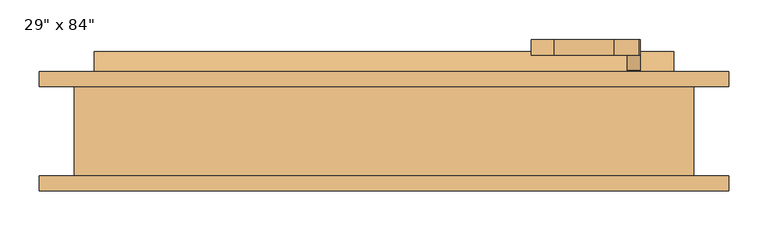
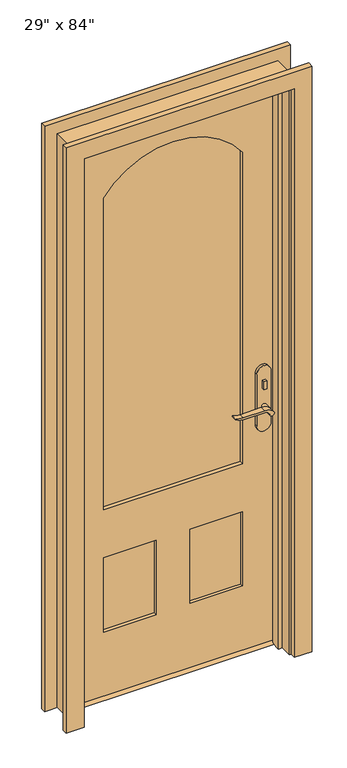
"""IFC4 building model written with IfcOpenShell, lengths in millimetres: door geometry."""

from ifc_helpers import new_model, si_unit, point, frame, frame_2d, origin, place, context, project, spatial, polyline, circle_curve, trimmed, segment, composite_curve, outline, extrude, faceted_brep, source, transform, mapped, element, save


def door_b81be692(model_context):
    return source(origin(), model_context, "Body", "SolidModel", [
        extrude(outline(polyline([(38.1, 12.7), (73.025, 12.7), (98.425, 0.0), (12.7, 0.0), (38.1, 12.7)])), frame((-368.3, 0.0, 0.0), z_axis=(1.0, 0.0, 0.0), x_axis=(0.0, 1.0, 0.0)), (0.0, 0.0, 1.0), 736.6),
        extrude(outline(polyline([(322.5, -0.95), (312.5, -0.95), (312.5, 9.05), (322.5, 9.05), (322.5, -0.95)])), frame((0.0, 0.0, 981.9), z_axis=(0.0, 0.0, 1.0), x_axis=(1.0, 0.0, 0.0)), (0.0, 0.0, 1.0), 30.0),
        extrude(outline(composite_curve([segment(trimmed(circle_curve(frame_2d((996.9, 317.5)), 8.0), [point((996.9, 309.5))], [point((996.9, 325.5))], False, "CARTESIAN"), True, "CONTINUOUS"), segment(trimmed(circle_curve(frame_2d((996.9, 317.5)), 8.0), [point((996.9, 325.5))], [point((996.9, 309.5))], False, "CARTESIAN"), True, "CONTINUOUS")], self_intersect=False)), frame((0.0, 63.975, 0.0), z_axis=(0.0, 1.0, 0.0), x_axis=(0.0, 0.0, 1.0)), (0.0, 0.0, 1.0), 10.0),
        extrude(outline(composite_curve([segment(trimmed(circle_curve(frame_2d((897.1555521, 293.8324871)), 37.2832219), [point((919.0523287, 324.0081363))], [point((934.4, 292.1325667))], False, "CARTESIAN"), True, "CONTINUOUS"), segment(polyline([(934.4, 292.1325667), (934.4, 215.8564091)]), True, "CONTINUOUS"), segment(trimmed(circle_curve(frame_2d((1017.6850638, 215.9227909)), 83.2850902), [point((934.4, 215.8564091))], [point((939.4, 187.5))], True, "CARTESIAN"), True, "CONTINUOUS"), segment(polyline([(939.4, 187.5), (936.6135558, 187.5)]), True, "CONTINUOUS"), segment(trimmed(circle_curve(frame_2d((986.6709207, 219.4396612)), 59.3791355), [point((936.6135558, 187.5))], [point((927.4, 215.8564091))], False, "CARTESIAN"), True, "CONTINUOUS"), segment(polyline([(927.4, 215.8564091), (927.4, 292.1138099)]), True, "CONTINUOUS"), segment(trimmed(circle_curve(frame_2d((909.2738613, 292.1138099)), 18.1261387), [point((927.4, 292.1138099))], [point((914.4, 309.5))], True, "CARTESIAN"), True, "CONTINUOUS"), segment(trimmed(circle_curve(frame_2d((914.4, 317.5)), 8.0), [point((914.4, 309.5))], [point((919.0523287, 324.0081363))], False, "CARTESIAN"), True, "CONTINUOUS")], self_intersect=False)), frame((0.0, -40.95, 0.0), z_axis=(0.0, 1.0, 0.0), x_axis=(0.0, 0.0, 1.0)), (0.0, 0.0, 1.0), 20.0),
        extrude(outline(composite_curve([segment(trimmed(circle_curve(frame_2d((914.4, 317.5)), 8.0), [point((914.3999903, 309.5))], [point((919.0523287, 324.0081363))], False, "CARTESIAN"), True, "CONTINUOUS"), segment(trimmed(circle_curve(frame_2d((897.1555521, 293.8324871)), 37.2832219), [point((919.0523287, 324.0081363))], [point((934.4, 292.1325667))], False, "CARTESIAN"), True, "CONTINUOUS"), segment(polyline([(934.4, 292.1325667), (934.4, 215.8564091)]), True, "CONTINUOUS"), segment(trimmed(circle_curve(frame_2d((1017.6850638, 215.9227909)), 83.2850902), [point((934.4, 215.8564091))], [point((939.4, 187.5))], True, "CARTESIAN"), True, "CONTINUOUS"), segment(polyline([(939.4, 187.5), (936.6135558, 187.5)]), True, "CONTINUOUS"), segment(trimmed(circle_curve(frame_2d((986.6709207, 219.4396612)), 59.3791355), [point((936.6135558, 187.5))], [point((927.4, 215.8564091))], False, "CARTESIAN"), True, "CONTINUOUS"), segment(polyline([(927.4, 215.8564091), (927.4, 292.1138122)]), True, "CONTINUOUS"), segment(trimmed(circle_curve(frame_2d((909.2738682, 292.1138122)), 18.1261318), [point((927.4, 292.1138122))], [point((914.3999903, 309.5))], True, "CARTESIAN"), True, "CONTINUOUS")], self_intersect=False)), frame((0.0, 93.975, 0.0), z_axis=(0.0, 1.0, 0.0), x_axis=(0.0, 0.0, 1.0)), (0.0, 0.0, 1.0), 20.0),
        extrude(outline(composite_curve([segment(trimmed(circle_curve(frame_2d((914.4, 317.5)), 8.0), [point((914.4, 309.5))], [point((914.4, 325.5))], False, "CARTESIAN"), True, "CONTINUOUS"), segment(trimmed(circle_curve(frame_2d((914.4, 317.5)), 8.0), [point((914.4, 325.5))], [point((914.4, 309.5))], False, "CARTESIAN"), True, "CONTINUOUS")], self_intersect=False)), frame((0.0, -20.95, 0.0), z_axis=(0.0, 1.0, 0.0), x_axis=(0.0, 0.0, 1.0)), (0.0, 0.0, 1.0), 30.0),
        extrude(outline(composite_curve([segment(trimmed(circle_curve(frame_2d((914.4, 317.5)), 8.0), [point((914.4, 309.5))], [point((914.4, 325.5))], False, "CARTESIAN"), True, "CONTINUOUS"), segment(trimmed(circle_curve(frame_2d((914.4, 317.5)), 8.0), [point((914.4, 325.5))], [point((914.4, 309.5))], False, "CARTESIAN"), True, "CONTINUOUS")], self_intersect=False)), frame((0.0, 63.975, 0.0), z_axis=(0.0, 1.0, 0.0), x_axis=(0.0, 0.0, 1.0)), (0.0, 0.0, 1.0), 30.0),
        extrude(outline(composite_curve([segment(polyline([(844.4, 342.5), (1039.4, 342.5)]), True, "CONTINUOUS"), segment(trimmed(circle_curve(frame_2d((1039.4, 317.5)), 25.0), [point((1039.4, 342.5))], [point((1039.4, 292.5))], False, "CARTESIAN"), True, "CONTINUOUS"), segment(polyline([(1039.4, 292.5), (844.4, 292.5)]), True, "CONTINUOUS"), segment(trimmed(circle_curve(frame_2d((844.4, 317.5)), 25.0), [point((844.4, 292.5))], [point((844.4, 342.5))], False, "CARTESIAN"), True, "CONTINUOUS")], self_intersect=False)), frame((0.0, 9.05, 0.0), z_axis=(0.0, 1.0, 0.0), x_axis=(0.0, 0.0, 1.0)), (0.0, 0.0, 1.0), 10.0),
        extrude(outline(composite_curve([segment(polyline([(844.4, 342.5), (1039.4, 342.5)]), True, "CONTINUOUS"), segment(trimmed(circle_curve(frame_2d((1039.4, 317.5)), 25.0), [point((1039.4, 342.5))], [point((1039.4, 292.5))], False, "CARTESIAN"), True, "CONTINUOUS"), segment(polyline([(1039.4, 292.5), (844.4, 292.5)]), True, "CONTINUOUS"), segment(trimmed(circle_curve(frame_2d((844.4, 317.5)), 25.0), [point((844.4, 292.5))], [point((844.4, 342.5))], False, "CARTESIAN"), True, "CONTINUOUS")], self_intersect=False)), frame((0.0, 53.975, 0.0), z_axis=(0.0, 1.0, 0.0), x_axis=(0.0, 0.0, 1.0)), (0.0, 0.0, 1.0), 10.0),
        faceted_brep([(393.7, 53.975, 0.0), (393.7, -60.325, 0.0), (368.3, -60.325, 0.0), (368.3, -15.875, 0.0), (355.6, -15.875, 0.0), (355.6, 19.05, 0.0), (368.3, 19.05, 0.0), (368.3, 53.975, 0.0), (393.7, 53.975, 2159.0), (393.7, -60.325, 2159.0), (-393.7, -60.325, 2159.0), (-393.7, -60.325, 0.0), (-368.3, -60.325, 0.0), (-368.3, -60.325, 2133.6), (368.3, -60.325, 2133.6), (368.3, -15.875, 2133.6), (-368.3, -15.875, 2133.6), (-368.3, -15.875, 0.0), (-355.6, -15.875, 0.0), (-355.6, -15.875, 2120.9), (355.6, -15.875, 2120.9), (355.6, 19.05, 2120.9), (-355.6, 19.05, 2120.9), (-355.6, 19.05, 0.0), (-368.3, 19.05, 0.0), (-368.3, 19.05, 2133.6), (368.3, 19.05, 2133.6), (368.3, 53.975, 2133.6), (-368.3, 53.975, 2133.6), (-368.3, 53.975, 0.0), (-393.7, 53.975, 0.0), (-393.7, 53.975, 2159.0)], [[[0, 1, 2, 3, 4, 5, 6, 7]], [[1, 0, 8, 9]], [[2, 1, 9, 10, 11, 12, 13, 14]], [[3, 2, 14, 15]], [[4, 3, 15, 16, 17, 18, 19, 20]], [[5, 4, 20, 21]], [[6, 5, 21, 22, 23, 24, 25, 26]], [[7, 6, 26, 27]], [[0, 7, 27, 28, 29, 30, 31, 8]], [[9, 8, 31, 10]], [[15, 14, 13, 16]], [[21, 20, 19, 22]], [[27, 26, 25, 28]], [[30, 29, 24, 23, 18, 17, 12, 11]], [[10, 31, 30, 11]], [[16, 13, 12, 17]], [[22, 19, 18, 23]], [[28, 25, 24, 29]]]),
        extrude(outline(polyline([(2133.6, -368.3), (12.7, -368.3), (12.7, 368.3), (2133.6, 368.3), (2133.6, -368.3)]), holes=[composite_curve([segment(polyline([(714.375, -247.65), (1885.95, -247.65)]), True, "CONTINUOUS"), segment(trimmed(circle_curve(frame_2d((1707.99125, 0.0)), 304.95875), [point((1885.95, -247.65))], [point((1885.95, 247.65))], True, "CARTESIAN"), True, "CONTINUOUS"), segment(polyline([(1885.95, 247.65), (714.375, 247.65), (714.375, -247.65)]), True, "CONTINUOUS")], self_intersect=False), polyline([(533.4, -60.325), (254.0, -60.325), (254.0, -247.65), (533.4, -247.65), (533.4, -60.325)]), polyline([(533.4, 247.65), (254.0, 247.65), (254.0, 60.325), (533.4, 60.325), (533.4, 247.65)])]), frame((0.0, 19.05, 0.0), z_axis=(0.0, 1.0, 0.0), x_axis=(0.0, 0.0, 1.0)), (0.0, 0.0, 1.0), 34.925),
        extrude(outline(composite_curve([segment(polyline([(714.375, -247.65), (714.375, 247.65), (1885.95, 247.65)]), True, "CONTINUOUS"), segment(trimmed(circle_curve(frame_2d((1707.99125, 0.0)), 304.95875), [point((1885.95, 247.65))], [point((1885.95, -247.65))], False, "CARTESIAN"), True, "CONTINUOUS"), segment(polyline([(1885.95, -247.65), (714.375, -247.65)]), True, "CONTINUOUS")], self_intersect=False)), frame((0.0, 33.02, 0.0), z_axis=(0.0, 1.0, 0.0), x_axis=(0.0, 0.0, 1.0)), (0.0, 0.0, 1.0), 6.985),
        extrude(outline(polyline([(-60.325, 30.6916667), (-247.65, 30.6916667), (-247.65, 42.3333333), (-60.325, 42.3333333), (-60.325, 30.6916667)])), frame((0.0, 0.0, 254.0), z_axis=(0.0, 0.0, 1.0), x_axis=(1.0, 0.0, 0.0)), (0.0, 0.0, 1.0), 279.4),
        extrude(outline(polyline([(247.65, 30.6916667), (60.325, 30.6916667), (60.325, 42.3333333), (247.65, 42.3333333), (247.65, 30.6916667)])), frame((0.0, 0.0, 254.0), z_axis=(0.0, 0.0, 1.0), x_axis=(1.0, 0.0, 0.0)), (0.0, 0.0, 1.0), 279.4),
        extrude(outline(polyline([(0.0, -438.15), (0.0, -374.65), (2139.95, -374.65), (2139.95, 374.65), (0.0, 374.65), (0.0, 438.15), (2203.45, 438.15), (2203.45, -438.15), (0.0, -438.15)])), frame((0.0, 53.975, 0.0), z_axis=(0.0, 1.0, 0.0), x_axis=(0.0, 0.0, 1.0)), (0.0, 0.0, 1.0), 19.05),
        extrude(outline(polyline([(0.0, -438.15), (0.0, -374.65), (2139.95, -374.65), (2139.95, 374.65), (0.0, 374.65), (0.0, 438.15), (2203.45, 438.15), (2203.45, -438.15), (0.0, -438.15)])), frame((0.0, -79.375, 0.0), z_axis=(0.0, 1.0, 0.0), x_axis=(0.0, 0.0, 1.0)), (0.0, 0.0, 1.0), 19.05),
    ])


if __name__ == "__main__":
    model = new_model("IFC4")
    model_context = context("Model", 3, world=origin())
    ifc_project = project(units=[si_unit("LENGTHUNIT", "METRE", prefix="MILLI")], contexts=[model_context])
    site = spatial("IfcSite", under=ifc_project)
    building = spatial("IfcBuilding", under=site)
    placement = place(None, origin())
    door_shape = door_b81be692(model_context)
    element("IfcDoor", 1, ObjectType="29\" x 84\"", at=placement, inside=building, context=model_context, shape_type="MappedRepresentation", body=[
        mapped(door_shape, transform((0.0, 0.0, 0.0), x_axis=(1.0, 0.0, 0.0), y_axis=(0.0, 1.0, 0.0), z_axis=(0.0, 0.0, 1.0))),
    ])
    save(model, "model.ifc")

# Revit data of these elements
# Type "29\" x 84\""
#   Type Mark = "8"
#   Assembly Code = "B2030100"
#   Analytic Construction = "French door, wood frame with single glass"
#   Threshold Offset [instance default] = 0' - 0 1/2"
#   Thickness = 0' - 1 3/8"
#   Thermal Resistance (R) = 1.0696 (h·ft²·°F)/BTU
#   Swing Angle [instance default] = 90.00°
#   Stiles = 0' - 4 3/4"
#   Rough Width = 2' - 7"
#   Rough Height = 7' - 1"
#   Radius = 1' - 0.00625"
#   Lock Rail = 0' - 7 1/8"
#   Height = 7' - 0"
#   Width = 2' - 5"
#   Heat Transfer Coefficient (U) = 0.9350 BTU/(h·ft²·°F)
#   Door Offset [instance default] = 0' - 0"
#   Bottom Rail = 0' - 9 1/2"
#   Threshold [instance default] = yes
#   Function = 1
#   Exterior Trim [instance default] = yes
#   Trim Material = Cherry
#   Threshold Material = Cherry
#   Panel Material = Cherry
#   Glazing = Glass
#   Frame Material = Cherry
#   Door Handle Material = Aluminum
#   Visual Light Transmittance = 0
#   Solar Heat Gain Coefficient = 0
#   Wall Closure = (empty or 0)
#   Construction Type = (empty or 0)
# Element 1 (IfcDoor, "29\" x 84\"")
#   Materials on its faces: "Cherry", "Aluminum", "Glass"
# Materials
#   "Cherry": class "Wood", colour RGB 226 177 128, transparency 0, Description = "Prunus Serotina", Cost = 0
#   "Glass": class "Glass", colour RGB 0 128 192, transparency 0.75, Description = "Soda Lime Glass", Cost = 0
#   "Aluminum": class "Metal", colour RGB 247 247 247, transparency 0, Description = "Aluminum 6061", Cost = 0
